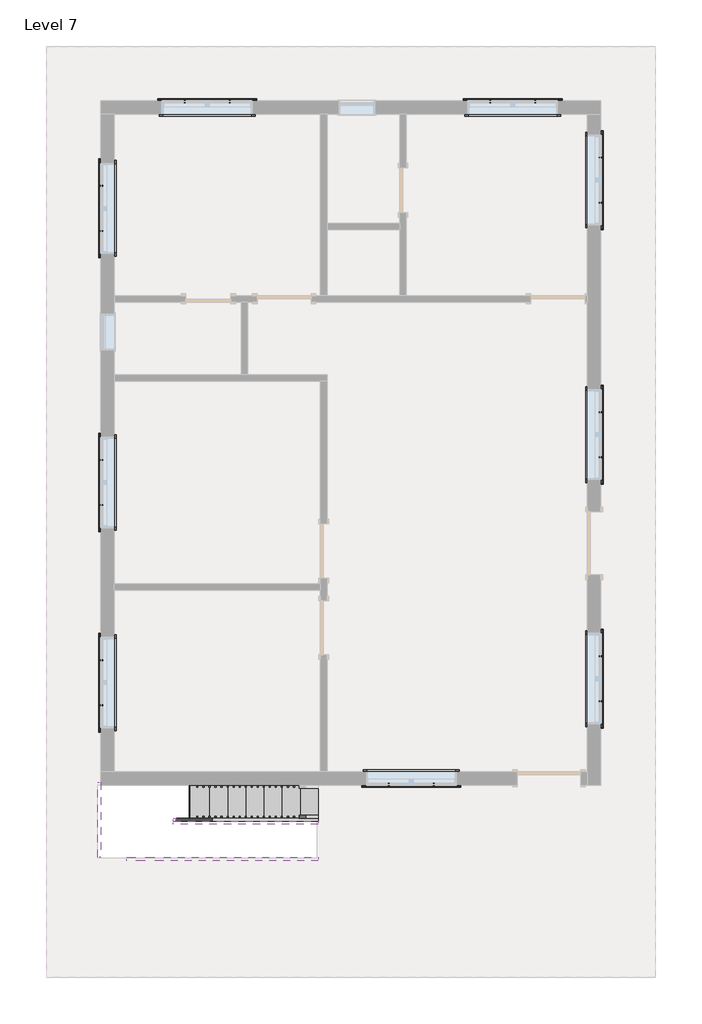
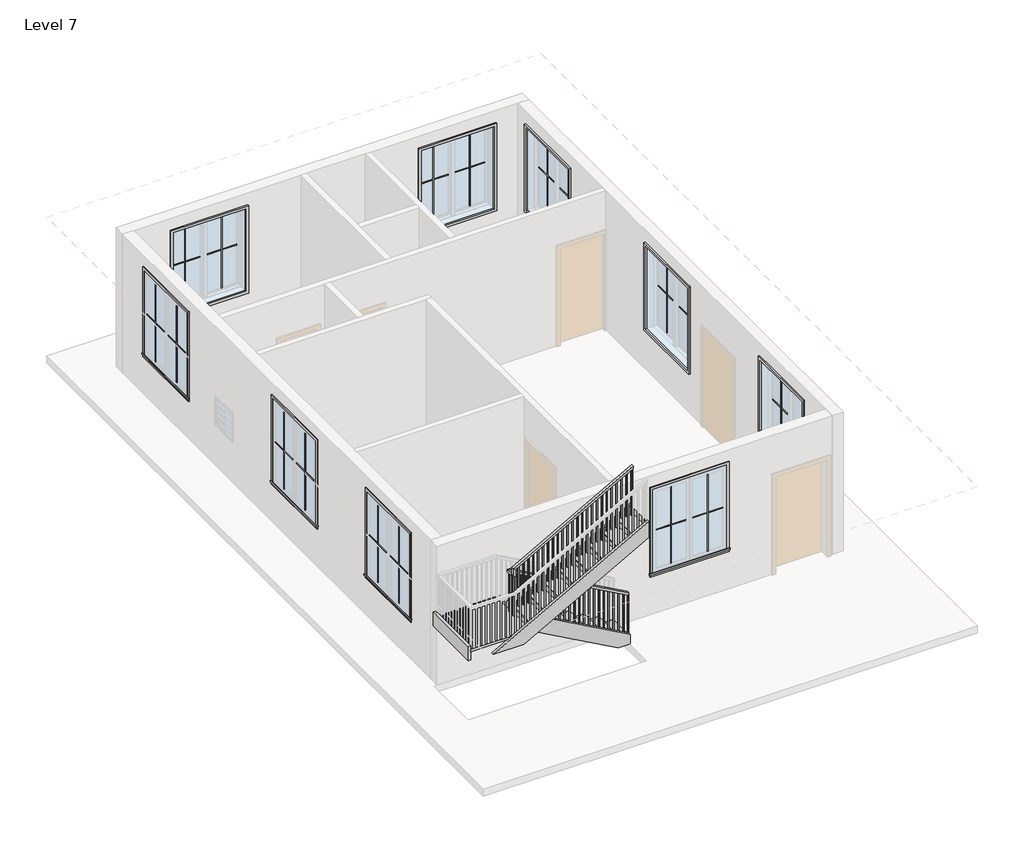
# One storey, part 3 of 3: 36 proxies, 6 members, 1 railing, 1 stair flight.
"""IFC4 building model written with IfcOpenShell, lengths in millimetres."""

from ifc_helpers import new_model, si_unit, frame, origin, place, context, project, spatial, polyline, outline, extrude, faceted_brep, transform, mapped, element, save
from components import muntin_pattern_2x2_muntin_pattern_2x2_f6a80940, muntin_pattern_2x2_muntin_pattern_2x2_09b00a1c, trim_window_exterior_flat_with_sill_698ed857, trim_window_interior_flat_picture_frame_92551a5e, stair_flight_b2054cc5

model = new_model("IFC4")

# Units and contexts
model_context = context("Model", 3, world=origin())
ifc_project = project(units=[si_unit("LENGTHUNIT", "METRE", prefix="MILLI")], contexts=[model_context])

# Site, building, storey
site = spatial("IfcSite", under=ifc_project)
building = spatial("IfcBuilding", under=site)
storey = spatial("IfcBuildingStorey", under=building, Name="Level 7", Elevation=16002.0)

# Proxies
placement = place(None, origin())
muntin_pattern_2x2_muntin_pattern_2x2_shape = muntin_pattern_2x2_muntin_pattern_2x2_f6a80940(model_context)
element("IfcBuildingElementProxy", 1, Name="Muntin Pattern_2x2 : Muntin Pattern_2x2", ObjectType="Muntin Pattern_2x2 : Muntin Pattern_2x2", at=placement, inside=storey, context=model_context, shape_type="MappedRepresentation", body=[
    mapped(muntin_pattern_2x2_muntin_pattern_2x2_shape, transform((-5453.9948569, -3961.7808037, 16986.25), x_axis=(0.0, 1.0, 0.0), y_axis=(-1.0, 0.0, 0.0), z_axis=(0.0, 0.0, 1.0))),
])
element("IfcBuildingElementProxy", 2, Name="Muntin Pattern_2x2 : Muntin Pattern_2x2", ObjectType="Muntin Pattern_2x2 : Muntin Pattern_2x2", at=placement, inside=storey, context=model_context, shape_type="MappedRepresentation", body=[
    mapped(muntin_pattern_2x2_muntin_pattern_2x2_shape, transform((-5453.9948569, -593.1058037, 16986.25), x_axis=(0.0, 1.0, 0.0), y_axis=(-1.0, 0.0, 0.0), z_axis=(0.0, 0.0, 1.0))),
])
element("IfcBuildingElementProxy", 3, Name="Muntin Pattern_2x2 : Muntin Pattern_2x2", ObjectType="Muntin Pattern_2x2 : Muntin Pattern_2x2", at=placement, inside=storey, context=model_context, shape_type="MappedRepresentation", body=[
    mapped(muntin_pattern_2x2_muntin_pattern_2x2_shape, transform((-5453.9948569, 4023.3441963, 16986.25), x_axis=(0.0, 1.0, 0.0), y_axis=(-1.0, 0.0, 0.0), z_axis=(0.0, 0.0, 1.0))),
])
element("IfcBuildingElementProxy", 4, Name="Muntin Pattern_2x2 : Muntin Pattern_2x2", ObjectType="Muntin Pattern_2x2 : Muntin Pattern_2x2", at=placement, inside=storey, context=model_context, shape_type="MappedRepresentation", body=[
    mapped(muntin_pattern_2x2_muntin_pattern_2x2_shape, transform((2947.0551431, 5258.4191963, 16986.25), x_axis=(0.0, -1.0, 0.0), y_axis=(1.0, 0.0, 0.0), z_axis=(0.0, 0.0, 1.0))),
])
element("IfcBuildingElementProxy", 5, Name="Muntin Pattern_2x2 : Muntin Pattern_2x2", ObjectType="Muntin Pattern_2x2 : Muntin Pattern_2x2", at=placement, inside=storey, context=model_context, shape_type="MappedRepresentation", body=[
    mapped(muntin_pattern_2x2_muntin_pattern_2x2_shape, transform((2947.0551431, 972.1691963, 16986.25), x_axis=(0.0, -1.0, 0.0), y_axis=(1.0, 0.0, 0.0), z_axis=(0.0, 0.0, 1.0))),
])
element("IfcBuildingElementProxy", 6, Name="Muntin Pattern_2x2 : Muntin Pattern_2x2", ObjectType="Muntin Pattern_2x2 : Muntin Pattern_2x2", at=placement, inside=storey, context=model_context, shape_type="MappedRepresentation", body=[
    mapped(muntin_pattern_2x2_muntin_pattern_2x2_shape, transform((2947.0551431, -3136.2808037, 16986.25), x_axis=(0.0, -1.0, 0.0), y_axis=(1.0, 0.0, 0.0), z_axis=(0.0, 0.0, 1.0))),
])
element("IfcBuildingElementProxy", 7, Name="Muntin Pattern_2x2 : Muntin Pattern_2x2", ObjectType="Muntin Pattern_2x2 : Muntin Pattern_2x2", at=placement, inside=storey, context=model_context, shape_type="MappedRepresentation", body=[
    mapped(muntin_pattern_2x2_muntin_pattern_2x2_shape, transform((141.9426431, -5296.8683037, 16986.25), x_axis=(-1.0, 0.0, 0.0), y_axis=(0.0, -1.0, 0.0), z_axis=(0.0, 0.0, 1.0))),
])
element("IfcBuildingElementProxy", 8, Name="Muntin Pattern_2x2 : Muntin Pattern_2x2", ObjectType="Muntin Pattern_2x2 : Muntin Pattern_2x2", at=placement, inside=storey, context=model_context, shape_type="MappedRepresentation", body=[
    mapped(muntin_pattern_2x2_muntin_pattern_2x2_shape, transform((1091.2676431, 6202.9816963, 16986.25), x_axis=(1.0, 0.0, 0.0), y_axis=(0.0, 1.0, 0.0), z_axis=(0.0, 0.0, 1.0))),
])
element("IfcBuildingElementProxy", 9, Name="Muntin Pattern_2x2 : Muntin Pattern_2x2", ObjectType="Muntin Pattern_2x2 : Muntin Pattern_2x2", at=placement, inside=storey, context=model_context, shape_type="MappedRepresentation", body=[
    mapped(muntin_pattern_2x2_muntin_pattern_2x2_shape, transform((-4052.2323569, 6202.9816963, 16986.25), x_axis=(1.0, 0.0, 0.0), y_axis=(0.0, 1.0, 0.0), z_axis=(0.0, 0.0, 1.0))),
])
muntin_pattern_2x2_muntin_pattern_2x2_2_shape = muntin_pattern_2x2_muntin_pattern_2x2_09b00a1c(model_context)
element("IfcBuildingElementProxy", 10, Name="Muntin Pattern_2x2 : Muntin Pattern_2x2", ObjectType="Muntin Pattern_2x2 : Muntin Pattern_2x2", at=placement, inside=storey, context=model_context, shape_type="MappedRepresentation", body=[
    mapped(muntin_pattern_2x2_muntin_pattern_2x2_2_shape, transform((-5453.9948569, -3202.9558037, 16986.25), x_axis=(0.0, -1.0, 0.0), y_axis=(1.0, 0.0, 0.0), z_axis=(0.0, 0.0, 1.0))),
])
element("IfcBuildingElementProxy", 11, Name="Muntin Pattern_2x2 : Muntin Pattern_2x2", ObjectType="Muntin Pattern_2x2 : Muntin Pattern_2x2", at=placement, inside=storey, context=model_context, shape_type="MappedRepresentation", body=[
    mapped(muntin_pattern_2x2_muntin_pattern_2x2_2_shape, transform((-5453.9948569, 165.7191963, 16986.25), x_axis=(0.0, -1.0, 0.0), y_axis=(1.0, 0.0, 0.0), z_axis=(0.0, 0.0, 1.0))),
])
element("IfcBuildingElementProxy", 12, Name="Muntin Pattern_2x2 : Muntin Pattern_2x2", ObjectType="Muntin Pattern_2x2 : Muntin Pattern_2x2", at=placement, inside=storey, context=model_context, shape_type="MappedRepresentation", body=[
    mapped(muntin_pattern_2x2_muntin_pattern_2x2_2_shape, transform((-5453.9948569, 4782.1691963, 16986.25), x_axis=(0.0, -1.0, 0.0), y_axis=(1.0, 0.0, 0.0), z_axis=(0.0, 0.0, 1.0))),
])
element("IfcBuildingElementProxy", 13, Name="Muntin Pattern_2x2 : Muntin Pattern_2x2", ObjectType="Muntin Pattern_2x2 : Muntin Pattern_2x2", at=placement, inside=storey, context=model_context, shape_type="MappedRepresentation", body=[
    mapped(muntin_pattern_2x2_muntin_pattern_2x2_2_shape, transform((2947.0551431, 4499.5941963, 16986.25), x_axis=(0.0, 1.0, 0.0), y_axis=(-1.0, 0.0, 0.0), z_axis=(0.0, 0.0, 1.0))),
])
element("IfcBuildingElementProxy", 14, Name="Muntin Pattern_2x2 : Muntin Pattern_2x2", ObjectType="Muntin Pattern_2x2 : Muntin Pattern_2x2", at=placement, inside=storey, context=model_context, shape_type="MappedRepresentation", body=[
    mapped(muntin_pattern_2x2_muntin_pattern_2x2_2_shape, transform((2947.0551431, 213.3441963, 16986.25), x_axis=(0.0, 1.0, 0.0), y_axis=(-1.0, 0.0, 0.0), z_axis=(0.0, 0.0, 1.0))),
])
element("IfcBuildingElementProxy", 15, Name="Muntin Pattern_2x2 : Muntin Pattern_2x2", ObjectType="Muntin Pattern_2x2 : Muntin Pattern_2x2", at=placement, inside=storey, context=model_context, shape_type="MappedRepresentation", body=[
    mapped(muntin_pattern_2x2_muntin_pattern_2x2_2_shape, transform((2947.0551431, -3895.1058037, 16986.25), x_axis=(0.0, 1.0, 0.0), y_axis=(-1.0, 0.0, 0.0), z_axis=(0.0, 0.0, 1.0))),
])
element("IfcBuildingElementProxy", 16, Name="Muntin Pattern_2x2 : Muntin Pattern_2x2", ObjectType="Muntin Pattern_2x2 : Muntin Pattern_2x2", at=placement, inside=storey, context=model_context, shape_type="MappedRepresentation", body=[
    mapped(muntin_pattern_2x2_muntin_pattern_2x2_2_shape, transform((-616.8823569, -5296.8683037, 16986.25), x_axis=(1.0, 0.0, 0.0), y_axis=(0.0, 1.0, 0.0), z_axis=(0.0, 0.0, 1.0))),
])
element("IfcBuildingElementProxy", 17, Name="Muntin Pattern_2x2 : Muntin Pattern_2x2", ObjectType="Muntin Pattern_2x2 : Muntin Pattern_2x2", at=placement, inside=storey, context=model_context, shape_type="MappedRepresentation", body=[
    mapped(muntin_pattern_2x2_muntin_pattern_2x2_2_shape, transform((1850.0926431, 6202.9816963, 16986.25), x_axis=(-1.0, 0.0, 0.0), y_axis=(0.0, -1.0, 0.0), z_axis=(0.0, 0.0, 1.0))),
])
element("IfcBuildingElementProxy", 18, Name="Muntin Pattern_2x2 : Muntin Pattern_2x2", ObjectType="Muntin Pattern_2x2 : Muntin Pattern_2x2", at=placement, inside=storey, context=model_context, shape_type="MappedRepresentation", body=[
    mapped(muntin_pattern_2x2_muntin_pattern_2x2_2_shape, transform((-3293.4073569, 6202.9816963, 16986.25), x_axis=(-1.0, 0.0, 0.0), y_axis=(0.0, -1.0, 0.0), z_axis=(0.0, 0.0, 1.0))),
])
trim_window_exterior_flat_with_sill_shape = trim_window_exterior_flat_with_sill_698ed857(model_context)
element("IfcBuildingElementProxy", 19, Name="Trim-Window-Exterior-Flat : with Sill", ObjectType="Trim-Window-Exterior-Flat : with Sill", at=placement, inside=storey, context=model_context, shape_type="MappedRepresentation", body=[
    mapped(trim_window_exterior_flat_with_sill_shape, transform((-5463.5198569, -3582.3683037, 18745.2), x_axis=(0.0, -1.0, 0.0), y_axis=(0.0, 0.0, 1.0), z_axis=(-1.0, 0.0, 0.0))),
])
element("IfcBuildingElementProxy", 20, Name="Trim-Window-Exterior-Flat : with Sill", ObjectType="Trim-Window-Exterior-Flat : with Sill", at=placement, inside=storey, context=model_context, shape_type="MappedRepresentation", body=[
    mapped(trim_window_exterior_flat_with_sill_shape, transform((-5463.5198569, -213.6933037, 18745.2), x_axis=(0.0, -1.0, 0.0), y_axis=(0.0, 0.0, 1.0), z_axis=(-1.0, 0.0, 0.0))),
])
element("IfcBuildingElementProxy", 21, Name="Trim-Window-Exterior-Flat : with Sill", ObjectType="Trim-Window-Exterior-Flat : with Sill", at=placement, inside=storey, context=model_context, shape_type="MappedRepresentation", body=[
    mapped(trim_window_exterior_flat_with_sill_shape, transform((-5463.5198569, 4402.7566963, 18745.2), x_axis=(0.0, -1.0, 0.0), y_axis=(0.0, 0.0, 1.0), z_axis=(-1.0, 0.0, 0.0))),
])
element("IfcBuildingElementProxy", 22, Name="Trim-Window-Exterior-Flat : with Sill", ObjectType="Trim-Window-Exterior-Flat : with Sill", at=placement, inside=storey, context=model_context, shape_type="MappedRepresentation", body=[
    mapped(trim_window_exterior_flat_with_sill_shape, transform((2956.5801431, 4879.0066963, 18745.2), x_axis=(0.0, 1.0, 0.0), y_axis=(0.0, 0.0, 1.0), z_axis=(1.0, 0.0, 0.0))),
])
element("IfcBuildingElementProxy", 23, Name="Trim-Window-Exterior-Flat : with Sill", ObjectType="Trim-Window-Exterior-Flat : with Sill", at=placement, inside=storey, context=model_context, shape_type="MappedRepresentation", body=[
    mapped(trim_window_exterior_flat_with_sill_shape, transform((2956.5801431, 592.7566963, 18745.2), x_axis=(0.0, 1.0, 0.0), y_axis=(0.0, 0.0, 1.0), z_axis=(1.0, 0.0, 0.0))),
])
element("IfcBuildingElementProxy", 24, Name="Trim-Window-Exterior-Flat : with Sill", ObjectType="Trim-Window-Exterior-Flat : with Sill", at=placement, inside=storey, context=model_context, shape_type="MappedRepresentation", body=[
    mapped(trim_window_exterior_flat_with_sill_shape, transform((2956.5801431, -3515.6933037, 18745.2), x_axis=(0.0, 1.0, 0.0), y_axis=(0.0, 0.0, 1.0), z_axis=(1.0, 0.0, 0.0))),
])
element("IfcBuildingElementProxy", 25, Name="Trim-Window-Exterior-Flat : with Sill", ObjectType="Trim-Window-Exterior-Flat : with Sill", at=placement, inside=storey, context=model_context, shape_type="MappedRepresentation", body=[
    mapped(trim_window_exterior_flat_with_sill_shape, transform((-237.4698569, -5306.3933037, 18745.2), x_axis=(1.0, 0.0, 0.0), y_axis=(0.0, 0.0, 1.0), z_axis=(0.0, -1.0, 0.0))),
])
element("IfcBuildingElementProxy", 26, Name="Trim-Window-Exterior-Flat : with Sill", ObjectType="Trim-Window-Exterior-Flat : with Sill", at=placement, inside=storey, context=model_context, shape_type="MappedRepresentation", body=[
    mapped(trim_window_exterior_flat_with_sill_shape, transform((1470.6801431, 6212.5066963, 18745.2), x_axis=(-1.0, 0.0, 0.0), y_axis=(0.0, 0.0, 1.0), z_axis=(0.0, 1.0, 0.0))),
])
element("IfcBuildingElementProxy", 27, Name="Trim-Window-Exterior-Flat : with Sill", ObjectType="Trim-Window-Exterior-Flat : with Sill", at=placement, inside=storey, context=model_context, shape_type="MappedRepresentation", body=[
    mapped(trim_window_exterior_flat_with_sill_shape, transform((-3672.8198569, 6212.5066963, 18745.2), x_axis=(-1.0, 0.0, 0.0), y_axis=(0.0, 0.0, 1.0), z_axis=(0.0, 1.0, 0.0))),
])
trim_window_interior_flat_picture_frame_shape = trim_window_interior_flat_picture_frame_92551a5e(model_context)
element("IfcBuildingElementProxy", 28, Name="Trim-Window-Interior-Flat : Picture Frame", ObjectType="Trim-Window-Interior-Flat : Picture Frame", at=placement, inside=storey, context=model_context, shape_type="MappedRepresentation", body=[
    mapped(trim_window_interior_flat_picture_frame_shape, transform((-5234.9198569, -3582.3683037, 18745.2), x_axis=(0.0, 1.0, 0.0), y_axis=(0.0, 0.0, 1.0), z_axis=(1.0, 0.0, 0.0))),
])
element("IfcBuildingElementProxy", 29, Name="Trim-Window-Interior-Flat : Picture Frame", ObjectType="Trim-Window-Interior-Flat : Picture Frame", at=placement, inside=storey, context=model_context, shape_type="MappedRepresentation", body=[
    mapped(trim_window_interior_flat_picture_frame_shape, transform((-5234.9198569, -213.6933037, 18745.2), x_axis=(0.0, 1.0, 0.0), y_axis=(0.0, 0.0, 1.0), z_axis=(1.0, 0.0, 0.0))),
])
element("IfcBuildingElementProxy", 30, Name="Trim-Window-Interior-Flat : Picture Frame", ObjectType="Trim-Window-Interior-Flat : Picture Frame", at=placement, inside=storey, context=model_context, shape_type="MappedRepresentation", body=[
    mapped(trim_window_interior_flat_picture_frame_shape, transform((-5234.9198569, 4402.7566963, 18745.2), x_axis=(0.0, 1.0, 0.0), y_axis=(0.0, 0.0, 1.0), z_axis=(1.0, 0.0, 0.0))),
])
element("IfcBuildingElementProxy", 31, Name="Trim-Window-Interior-Flat : Picture Frame", ObjectType="Trim-Window-Interior-Flat : Picture Frame", at=placement, inside=storey, context=model_context, shape_type="MappedRepresentation", body=[
    mapped(trim_window_interior_flat_picture_frame_shape, transform((2727.9801431, 4879.0066963, 18745.2), x_axis=(0.0, -1.0, 0.0), y_axis=(0.0, 0.0, 1.0), z_axis=(-1.0, 0.0, 0.0))),
])
element("IfcBuildingElementProxy", 32, Name="Trim-Window-Interior-Flat : Picture Frame", ObjectType="Trim-Window-Interior-Flat : Picture Frame", at=placement, inside=storey, context=model_context, shape_type="MappedRepresentation", body=[
    mapped(trim_window_interior_flat_picture_frame_shape, transform((2727.9801431, 592.7566963, 18745.2), x_axis=(0.0, -1.0, 0.0), y_axis=(0.0, 0.0, 1.0), z_axis=(-1.0, 0.0, 0.0))),
])
element("IfcBuildingElementProxy", 33, Name="Trim-Window-Interior-Flat : Picture Frame", ObjectType="Trim-Window-Interior-Flat : Picture Frame", at=placement, inside=storey, context=model_context, shape_type="MappedRepresentation", body=[
    mapped(trim_window_interior_flat_picture_frame_shape, transform((2727.9801431, -3515.6933037, 18745.2), x_axis=(0.0, -1.0, 0.0), y_axis=(0.0, 0.0, 1.0), z_axis=(-1.0, 0.0, 0.0))),
])
element("IfcBuildingElementProxy", 34, Name="Trim-Window-Interior-Flat : Picture Frame", ObjectType="Trim-Window-Interior-Flat : Picture Frame", at=placement, inside=storey, context=model_context, shape_type="MappedRepresentation", body=[
    mapped(trim_window_interior_flat_picture_frame_shape, transform((-237.4698569, -5077.7933037, 18745.2), x_axis=(-1.0, 0.0, 0.0), y_axis=(0.0, 0.0, 1.0), z_axis=(0.0, 1.0, 0.0))),
])
element("IfcBuildingElementProxy", 35, Name="Trim-Window-Interior-Flat : Picture Frame", ObjectType="Trim-Window-Interior-Flat : Picture Frame", at=placement, inside=storey, context=model_context, shape_type="MappedRepresentation", body=[
    mapped(trim_window_interior_flat_picture_frame_shape, transform((1470.6801431, 5983.9066963, 18745.2), x_axis=(1.0, 0.0, 0.0), y_axis=(0.0, 0.0, 1.0), z_axis=(0.0, -1.0, 0.0))),
])
element("IfcBuildingElementProxy", 36, Name="Trim-Window-Interior-Flat : Picture Frame", ObjectType="Trim-Window-Interior-Flat : Picture Frame", at=placement, inside=storey, context=model_context, shape_type="MappedRepresentation", body=[
    mapped(trim_window_interior_flat_picture_frame_shape, transform((-3672.8198569, 5983.9066963, 18745.2), x_axis=(1.0, 0.0, 0.0), y_axis=(0.0, 0.0, 1.0), z_axis=(0.0, -1.0, 0.0))),
])

# Members
element("IfcMember", 37, ObjectType="Stringer - 2\" Width", at=placement, inside=storey, context=model_context, shape_type="SweptSolid", body=[
    extrude(outline(polyline([(16002.0, -1805.9198569), (16209.5983948, -1805.9198569), (17536.0428392, -4193.5198569), (17187.3641651, -4193.5198569), (16002.0, -2059.8643597), (16002.0, -1805.9198569)])), frame((0.0, -5915.9933037, 0.0), z_axis=(0.0, 1.0, 0.0), x_axis=(0.0, 0.0, 1.0)), (0.0, 0.0, 1.0), 50.8),
])
element("IfcMember", 38, ObjectType="Stringer - 2\" Width", at=placement, inside=storey, context=model_context, shape_type="SweptSolid", body=[
    extrude(outline(polyline([(-4244.3198569, -5865.1933037), (-4193.5198569, -5865.1933037), (-4193.5198569, -5915.9933037), (-4244.3198569, -5915.9933037), (-4244.3198569, -5865.1933037)])), frame((0.0, 0.0, 17297.4), z_axis=(0.0, 0.0, 1.0), x_axis=(1.0, 0.0, 0.0)), (0.0, 0.0, 1.0), 304.8),
])
element("IfcMember", 39, ObjectType="Stringer - 2\" Width", at=placement, inside=storey, context=model_context, shape_type="SweptSolid", body=[
    extrude(outline(polyline([(17733.5983948, -4244.3198569), (17384.9197207, -4244.3198569), (18739.5863873, -1805.9198569), (19088.2650614, -1805.9198569), (17733.5983948, -4244.3198569)])), frame((0.0, -5966.7933037, 0.0), z_axis=(0.0, 1.0, 0.0), x_axis=(0.0, 0.0, 1.0)), (0.0, 0.0, 1.0), 50.8),
])
element("IfcMember", 40, ObjectType="Stringer - 2\" Width", at=placement, inside=storey, context=model_context, shape_type="SweptSolid", body=[
    extrude(outline(polyline([(16002.0, -1805.9198569), (16209.5983948, -1805.9198569), (17602.2, -4312.6027463), (17602.2, -4940.2243597), (16002.0, -2059.8643597), (16002.0, -1805.9198569)])), frame((0.0, -5306.3933037, 0.0), z_axis=(0.0, 1.0, 0.0), x_axis=(0.0, 0.0, 1.0)), (0.0, 0.0, 1.0), 50.8),
])
element("IfcMember", 41, ObjectType="Stringer - 2\" Width", at=placement, inside=storey, context=model_context, shape_type="SweptSolid", body=[
    extrude(outline(polyline([(-5514.3198569, -5255.5933037), (-5463.5198569, -5255.5933037), (-5463.5198569, -6525.5933037), (-5514.3198569, -6525.5933037), (-5514.3198569, -5255.5933037)])), frame((0.0, 0.0, 17297.4), z_axis=(0.0, 0.0, 1.0), x_axis=(1.0, 0.0, 0.0)), (0.0, 0.0, 1.0), 304.8),
])
element("IfcMember", 42, ObjectType="Stringer - 2\" Width", at=placement, inside=storey, context=model_context, shape_type="SweptSolid", body=[
    extrude(outline(polyline([(17297.4, -4401.8553541), (18739.5863873, -1805.9198569), (19088.2650614, -1805.9198569), (17297.4, -5029.4769675), (17297.4, -4401.8553541)])), frame((0.0, -6576.3933037, 0.0), z_axis=(0.0, 1.0, 0.0), x_axis=(0.0, 0.0, 1.0)), (0.0, 0.0, 1.0), 50.8),
])

# Railing
element("IfcRailing", 43, ObjectType="Handrail - Rectangular", at=placement, inside=storey, context=model_context, shape_type="SolidModel", body=[
    faceted_brep([(-1805.9198569, -5865.1933037, 17085.7333333), (-1805.9198569, -5865.1933037, 17027.620221), (-1805.9198569, -5814.3933037, 17027.620221), (-1805.9198569, -5814.3933037, 17085.7333333), (-4168.1198569, -5865.1933037, 18398.0666667), (-4218.9198569, -5865.1933037, 18368.1757765), (-4218.9198569, -5814.3933037, 18368.1757765), (-4168.1198569, -5814.3933037, 18398.0666667), (-4168.1198569, -5865.1933037, 18440.4), (-4218.9198569, -5865.1933037, 18389.6), (-4218.9198569, -5814.3933037, 18389.6), (-4168.1198569, -5814.3933037, 18440.4), (-4244.3198569, -5865.1933037, 18440.4), (-4244.3198569, -5865.1933037, 18389.6), (-4295.1198569, -5814.3933037, 18389.6), (-4295.1198569, -5814.3933037, 18440.4), (-4244.3198569, -5941.3933037, 18440.4), (-4244.3198569, -5941.3933037, 18389.6), (-4295.1198569, -5941.3933037, 18389.6), (-4295.1198569, -5941.3933037, 18440.4), (-4244.3198569, -5966.7933037, 18440.4), (-4295.1198569, -5966.7933037, 18440.4), (-4295.1198569, -6017.5933037, 18389.6), (-4244.3198569, -6017.5933037, 18389.6)], [[[0, 1, 2, 3]], [[1, 0, 4, 5]], [[2, 1, 5, 6]], [[3, 2, 6, 7]], [[0, 3, 7, 4]], [[5, 4, 8, 9]], [[6, 5, 9, 10]], [[7, 6, 10, 11]], [[4, 7, 11, 8]], [[9, 8, 12, 13]], [[10, 9, 13, 14]], [[11, 10, 14, 15]], [[8, 11, 15, 12]], [[13, 12, 16, 17]], [[14, 13, 17, 18]], [[15, 14, 18, 19]], [[12, 15, 19, 16]], [[20, 21, 22, 23]], [[17, 16, 20, 23]], [[18, 17, 23, 22]], [[19, 18, 22, 21]], [[16, 19, 21, 20]]]),
    faceted_brep([(-4244.3198569, -5966.7933037, 18440.4), (-4244.3198569, -6017.5933037, 18389.6), (-4295.1198569, -6017.5933037, 18389.6), (-4295.1198569, -5966.7933037, 18440.4), (-4244.3198569, -5966.7933037, 18551.620221), (-4295.1198569, -5966.7933037, 18581.5111111), (-4295.1198569, -6017.5933037, 18581.5111111), (-4244.3198569, -6017.5933037, 18551.620221)], [[[0, 1, 2, 3]], [[4, 5, 6, 7]], [[1, 0, 4, 7]], [[2, 1, 7, 6]], [[3, 2, 6, 5]], [[0, 3, 5, 4]]]),
    faceted_brep([(-4295.1198569, -5966.7933037, 18581.5111111), (-4244.3198569, -5966.7933037, 18551.620221), (-4244.3198569, -6017.5933037, 18551.620221), (-4295.1198569, -6017.5933037, 18581.5111111), (-1805.9198569, -5966.7933037, 19964.4), (-1805.9198569, -6017.5933037, 19964.4), (-1805.9198569, -6017.5933037, 19906.2868876), (-1805.9198569, -5966.7933037, 19906.2868876)], [[[0, 1, 2, 3]], [[4, 5, 6, 7]], [[1, 0, 4, 7]], [[2, 1, 7, 6]], [[3, 2, 6, 5]], [[0, 3, 5, 4]]]),
    extrude(outline(polyline([(19886.8841099, -1840.8448569), (18880.6666667, -1840.8448569), (18880.6666667, -1821.7948569), (19897.4674432, -1821.7948569), (19886.8841099, -1840.8448569)])), frame((0.0, -6001.7183037, 0.0), z_axis=(0.0, 1.0, 0.0), x_axis=(0.0, 0.0, 1.0)), (0.0, 0.0, 1.0), 19.05),
    extrude(outline(polyline([(19830.4396654, -1942.4448569), (18880.6666667, -1942.4448569), (18880.6666667, -1923.3948569), (19841.0229988, -1923.3948569), (19830.4396654, -1942.4448569)])), frame((0.0, -6001.7183037, 0.0), z_axis=(0.0, 1.0, 0.0), x_axis=(0.0, 0.0, 1.0)), (0.0, 0.0, 1.0), 19.05),
    extrude(outline(polyline([(19773.995221, -2044.0448569), (18880.6666667, -2044.0448569), (18880.6666667, -2024.9948569), (19784.5785543, -2024.9948569), (19773.995221, -2044.0448569)])), frame((0.0, -6001.7183037, 0.0), z_axis=(0.0, 1.0, 0.0), x_axis=(0.0, 0.0, 1.0)), (0.0, 0.0, 1.0), 19.05),
    extrude(outline(polyline([(19717.5507765, -2145.6448569), (18711.3333333, -2145.6448569), (18711.3333333, -2126.5948569), (19728.1341099, -2126.5948569), (19717.5507765, -2145.6448569)])), frame((0.0, -6001.7183037, 0.0), z_axis=(0.0, 1.0, 0.0), x_axis=(0.0, 0.0, 1.0)), (0.0, 0.0, 1.0), 19.05),
    extrude(outline(polyline([(19661.1063321, -2247.2448569), (18711.3333333, -2247.2448569), (18711.3333333, -2228.1948569), (19671.6896654, -2228.1948569), (19661.1063321, -2247.2448569)])), frame((0.0, -6001.7183037, 0.0), z_axis=(0.0, 1.0, 0.0), x_axis=(0.0, 0.0, 1.0)), (0.0, 0.0, 1.0), 19.05),
    extrude(outline(polyline([(19604.6618876, -2348.8448569), (18711.3333333, -2348.8448569), (18711.3333333, -2329.7948569), (19615.245221, -2329.7948569), (19604.6618876, -2348.8448569)])), frame((0.0, -6001.7183037, 0.0), z_axis=(0.0, 1.0, 0.0), x_axis=(0.0, 0.0, 1.0)), (0.0, 0.0, 1.0), 19.05),
    extrude(outline(polyline([(19548.2174432, -2450.4448569), (18542.0, -2450.4448569), (18542.0, -2431.3948569), (19558.8007765, -2431.3948569), (19548.2174432, -2450.4448569)])), frame((0.0, -6001.7183037, 0.0), z_axis=(0.0, 1.0, 0.0), x_axis=(0.0, 0.0, 1.0)), (0.0, 0.0, 1.0), 19.05),
    extrude(outline(polyline([(19491.7729988, -2552.0448569), (18542.0, -2552.0448569), (18542.0, -2532.9948569), (19502.3563321, -2532.9948569), (19491.7729988, -2552.0448569)])), frame((0.0, -6001.7183037, 0.0), z_axis=(0.0, 1.0, 0.0), x_axis=(0.0, 0.0, 1.0)), (0.0, 0.0, 1.0), 19.05),
    extrude(outline(polyline([(19435.3285543, -2653.6448569), (18542.0, -2653.6448569), (18542.0, -2634.5948569), (19445.9118876, -2634.5948569), (19435.3285543, -2653.6448569)])), frame((0.0, -6001.7183037, 0.0), z_axis=(0.0, 1.0, 0.0), x_axis=(0.0, 0.0, 1.0)), (0.0, 0.0, 1.0), 19.05),
    extrude(outline(polyline([(19378.8841099, -2755.2448569), (18372.6666667, -2755.2448569), (18372.6666667, -2736.1948569), (19389.4674432, -2736.1948569), (19378.8841099, -2755.2448569)])), frame((0.0, -6001.7183037, 0.0), z_axis=(0.0, 1.0, 0.0), x_axis=(0.0, 0.0, 1.0)), (0.0, 0.0, 1.0), 19.05),
    extrude(outline(polyline([(19322.4396654, -2856.8448569), (18372.6666667, -2856.8448569), (18372.6666667, -2837.7948569), (19333.0229988, -2837.7948569), (19322.4396654, -2856.8448569)])), frame((0.0, -6001.7183037, 0.0), z_axis=(0.0, 1.0, 0.0), x_axis=(0.0, 0.0, 1.0)), (0.0, 0.0, 1.0), 19.05),
    extrude(outline(polyline([(19265.995221, -2958.4448569), (18372.6666667, -2958.4448569), (18372.6666667, -2939.3948569), (19276.5785543, -2939.3948569), (19265.995221, -2958.4448569)])), frame((0.0, -6001.7183037, 0.0), z_axis=(0.0, 1.0, 0.0), x_axis=(0.0, 0.0, 1.0)), (0.0, 0.0, 1.0), 19.05),
    extrude(outline(polyline([(19209.5507765, -3060.0448569), (18203.3333333, -3060.0448569), (18203.3333333, -3040.9948569), (19220.1341099, -3040.9948569), (19209.5507765, -3060.0448569)])), frame((0.0, -6001.7183037, 0.0), z_axis=(0.0, 1.0, 0.0), x_axis=(0.0, 0.0, 1.0)), (0.0, 0.0, 1.0), 19.05),
    extrude(outline(polyline([(19153.1063321, -3161.6448569), (18203.3333333, -3161.6448569), (18203.3333333, -3142.5948569), (19163.6896654, -3142.5948569), (19153.1063321, -3161.6448569)])), frame((0.0, -6001.7183037, 0.0), z_axis=(0.0, 1.0, 0.0), x_axis=(0.0, 0.0, 1.0)), (0.0, 0.0, 1.0), 19.05),
    extrude(outline(polyline([(19096.6618876, -3263.2448569), (18203.3333333, -3263.2448569), (18203.3333333, -3244.1948569), (19107.245221, -3244.1948569), (19096.6618876, -3263.2448569)])), frame((0.0, -6001.7183037, 0.0), z_axis=(0.0, 1.0, 0.0), x_axis=(0.0, 0.0, 1.0)), (0.0, 0.0, 1.0), 19.05),
    extrude(outline(polyline([(19040.2174432, -3364.8448569), (18034.0, -3364.8448569), (18034.0, -3345.7948569), (19050.8007765, -3345.7948569), (19040.2174432, -3364.8448569)])), frame((0.0, -6001.7183037, 0.0), z_axis=(0.0, 1.0, 0.0), x_axis=(0.0, 0.0, 1.0)), (0.0, 0.0, 1.0), 19.05),
    extrude(outline(polyline([(18983.7729988, -3466.4448569), (18034.0, -3466.4448569), (18034.0, -3447.3948569), (18994.3563321, -3447.3948569), (18983.7729988, -3466.4448569)])), frame((0.0, -6001.7183037, 0.0), z_axis=(0.0, 1.0, 0.0), x_axis=(0.0, 0.0, 1.0)), (0.0, 0.0, 1.0), 19.05),
    extrude(outline(polyline([(18927.3285543, -3568.0448569), (18034.0, -3568.0448569), (18034.0, -3548.9948569), (18937.9118876, -3548.9948569), (18927.3285543, -3568.0448569)])), frame((0.0, -6001.7183037, 0.0), z_axis=(0.0, 1.0, 0.0), x_axis=(0.0, 0.0, 1.0)), (0.0, 0.0, 1.0), 19.05),
    extrude(outline(polyline([(18870.8841099, -3669.6448569), (17864.6666667, -3669.6448569), (17864.6666667, -3650.5948569), (18881.4674432, -3650.5948569), (18870.8841099, -3669.6448569)])), frame((0.0, -6001.7183037, 0.0), z_axis=(0.0, 1.0, 0.0), x_axis=(0.0, 0.0, 1.0)), (0.0, 0.0, 1.0), 19.05),
    extrude(outline(polyline([(18814.4396654, -3771.2448569), (17864.6666667, -3771.2448569), (17864.6666667, -3752.1948569), (18825.0229988, -3752.1948569), (18814.4396654, -3771.2448569)])), frame((0.0, -6001.7183037, 0.0), z_axis=(0.0, 1.0, 0.0), x_axis=(0.0, 0.0, 1.0)), (0.0, 0.0, 1.0), 19.05),
    extrude(outline(polyline([(18757.995221, -3872.8448569), (17864.6666667, -3872.8448569), (17864.6666667, -3853.7948569), (18768.5785543, -3853.7948569), (18757.995221, -3872.8448569)])), frame((0.0, -6001.7183037, 0.0), z_axis=(0.0, 1.0, 0.0), x_axis=(0.0, 0.0, 1.0)), (0.0, 0.0, 1.0), 19.05),
    extrude(outline(polyline([(18701.5507765, -3974.4448569), (17695.3333333, -3974.4448569), (17695.3333333, -3955.3948569), (18712.1341099, -3955.3948569), (18701.5507765, -3974.4448569)])), frame((0.0, -6001.7183037, 0.0), z_axis=(0.0, 1.0, 0.0), x_axis=(0.0, 0.0, 1.0)), (0.0, 0.0, 1.0), 19.05),
    extrude(outline(polyline([(18645.1063321, -4076.0448569), (17695.3333333, -4076.0448569), (17695.3333333, -4056.9948569), (18655.6896654, -4056.9948569), (18645.1063321, -4076.0448569)])), frame((0.0, -6001.7183037, 0.0), z_axis=(0.0, 1.0, 0.0), x_axis=(0.0, 0.0, 1.0)), (0.0, 0.0, 1.0), 19.05),
    extrude(outline(polyline([(18588.6618876, -4177.6448569), (17695.3333333, -4177.6448569), (17695.3333333, -4158.5948569), (18599.245221, -4158.5948569), (18588.6618876, -4177.6448569)])), frame((0.0, -6001.7183037, 0.0), z_axis=(0.0, 1.0, 0.0), x_axis=(0.0, 0.0, 1.0)), (0.0, 0.0, 1.0), 19.05),
    extrude(outline(polyline([(-4260.1948569, -5931.8683037), (-4260.1948569, -5950.9183037), (-4279.2448569, -5950.9183037), (-4279.2448569, -5931.8683037), (-4260.1948569, -5931.8683037)])), frame((0.0, 0.0, 17526.0), z_axis=(0.0, 0.0, 1.0), x_axis=(1.0, 0.0, 0.0)), (0.0, 0.0, 1.0), 863.6),
    extrude(outline(polyline([(-4234.7948569, -5849.3183037), (-4253.8448569, -5849.3183037), (-4253.8448569, -5830.2683037), (-4234.7948569, -5830.2683037), (-4234.7948569, -5849.3183037)])), frame((0.0, 0.0, 17526.0), z_axis=(0.0, 0.0, 1.0), x_axis=(1.0, 0.0, 0.0)), (0.0, 0.0, 1.0), 863.6),
    extrude(outline(polyline([(18331.1341099, -4152.2448569), (17356.6666667, -4152.2448569), (17356.6666667, -4133.1948569), (18320.5507765, -4133.1948569), (18331.1341099, -4152.2448569)])), frame((0.0, -5849.3183037, 0.0), z_axis=(0.0, 1.0, 0.0), x_axis=(0.0, 0.0, 1.0)), (0.0, 0.0, 1.0), 19.05),
    extrude(outline(polyline([(18274.6896654, -4050.6448569), (17356.6666667, -4050.6448569), (17356.6666667, -4031.5948569), (18264.1063321, -4031.5948569), (18274.6896654, -4050.6448569)])), frame((0.0, -5849.3183037, 0.0), z_axis=(0.0, 1.0, 0.0), x_axis=(0.0, 0.0, 1.0)), (0.0, 0.0, 1.0), 19.05),
    extrude(outline(polyline([(18218.245221, -3949.0448569), (17356.6666667, -3949.0448569), (17356.6666667, -3929.9948569), (18207.6618876, -3929.9948569), (18218.245221, -3949.0448569)])), frame((0.0, -5849.3183037, 0.0), z_axis=(0.0, 1.0, 0.0), x_axis=(0.0, 0.0, 1.0)), (0.0, 0.0, 1.0), 19.05),
    extrude(outline(polyline([(18161.8007765, -3847.4448569), (17187.3333333, -3847.4448569), (17187.3333333, -3828.3948569), (18151.2174432, -3828.3948569), (18161.8007765, -3847.4448569)])), frame((0.0, -5849.3183037, 0.0), z_axis=(0.0, 1.0, 0.0), x_axis=(0.0, 0.0, 1.0)), (0.0, 0.0, 1.0), 19.05),
    extrude(outline(polyline([(18105.3563321, -3745.8448569), (17187.3333333, -3745.8448569), (17187.3333333, -3726.7948569), (18094.7729988, -3726.7948569), (18105.3563321, -3745.8448569)])), frame((0.0, -5849.3183037, 0.0), z_axis=(0.0, 1.0, 0.0), x_axis=(0.0, 0.0, 1.0)), (0.0, 0.0, 1.0), 19.05),
    extrude(outline(polyline([(18048.9118876, -3644.2448569), (17187.3333333, -3644.2448569), (17187.3333333, -3625.1948569), (18038.3285543, -3625.1948569), (18048.9118876, -3644.2448569)])), frame((0.0, -5849.3183037, 0.0), z_axis=(0.0, 1.0, 0.0), x_axis=(0.0, 0.0, 1.0)), (0.0, 0.0, 1.0), 19.05),
    extrude(outline(polyline([(17992.4674432, -3542.6448569), (17018.0, -3542.6448569), (17018.0, -3523.5948569), (17981.8841099, -3523.5948569), (17992.4674432, -3542.6448569)])), frame((0.0, -5849.3183037, 0.0), z_axis=(0.0, 1.0, 0.0), x_axis=(0.0, 0.0, 1.0)), (0.0, 0.0, 1.0), 19.05),
    extrude(outline(polyline([(17936.0229988, -3441.0448569), (17018.0, -3441.0448569), (17018.0, -3421.9948569), (17925.4396654, -3421.9948569), (17936.0229988, -3441.0448569)])), frame((0.0, -5849.3183037, 0.0), z_axis=(0.0, 1.0, 0.0), x_axis=(0.0, 0.0, 1.0)), (0.0, 0.0, 1.0), 19.05),
    extrude(outline(polyline([(17879.5785543, -3339.4448569), (17018.0, -3339.4448569), (17018.0, -3320.3948569), (17868.995221, -3320.3948569), (17879.5785543, -3339.4448569)])), frame((0.0, -5849.3183037, 0.0), z_axis=(0.0, 1.0, 0.0), x_axis=(0.0, 0.0, 1.0)), (0.0, 0.0, 1.0), 19.05),
    extrude(outline(polyline([(17823.1341099, -3237.8448569), (16848.6666667, -3237.8448569), (16848.6666667, -3218.7948569), (17812.5507765, -3218.7948569), (17823.1341099, -3237.8448569)])), frame((0.0, -5849.3183037, 0.0), z_axis=(0.0, 1.0, 0.0), x_axis=(0.0, 0.0, 1.0)), (0.0, 0.0, 1.0), 19.05),
    extrude(outline(polyline([(17766.6896654, -3136.2448569), (16848.6666667, -3136.2448569), (16848.6666667, -3117.1948569), (17756.1063321, -3117.1948569), (17766.6896654, -3136.2448569)])), frame((0.0, -5849.3183037, 0.0), z_axis=(0.0, 1.0, 0.0), x_axis=(0.0, 0.0, 1.0)), (0.0, 0.0, 1.0), 19.05),
    extrude(outline(polyline([(17710.245221, -3034.6448569), (16848.6666667, -3034.6448569), (16848.6666667, -3015.5948569), (17699.6618876, -3015.5948569), (17710.245221, -3034.6448569)])), frame((0.0, -5849.3183037, 0.0), z_axis=(0.0, 1.0, 0.0), x_axis=(0.0, 0.0, 1.0)), (0.0, 0.0, 1.0), 19.05),
    extrude(outline(polyline([(17653.8007765, -2933.0448569), (16679.3333333, -2933.0448569), (16679.3333333, -2913.9948569), (17643.2174432, -2913.9948569), (17653.8007765, -2933.0448569)])), frame((0.0, -5849.3183037, 0.0), z_axis=(0.0, 1.0, 0.0), x_axis=(0.0, 0.0, 1.0)), (0.0, 0.0, 1.0), 19.05),
    extrude(outline(polyline([(17597.3563321, -2831.4448569), (16679.3333333, -2831.4448569), (16679.3333333, -2812.3948569), (17586.7729988, -2812.3948569), (17597.3563321, -2831.4448569)])), frame((0.0, -5849.3183037, 0.0), z_axis=(0.0, 1.0, 0.0), x_axis=(0.0, 0.0, 1.0)), (0.0, 0.0, 1.0), 19.05),
    extrude(outline(polyline([(17540.9118876, -2729.8448569), (16679.3333333, -2729.8448569), (16679.3333333, -2710.7948569), (17530.3285543, -2710.7948569), (17540.9118876, -2729.8448569)])), frame((0.0, -5849.3183037, 0.0), z_axis=(0.0, 1.0, 0.0), x_axis=(0.0, 0.0, 1.0)), (0.0, 0.0, 1.0), 19.05),
    extrude(outline(polyline([(17484.4674432, -2628.2448569), (16510.0, -2628.2448569), (16510.0, -2609.1948569), (17473.8841099, -2609.1948569), (17484.4674432, -2628.2448569)])), frame((0.0, -5849.3183037, 0.0), z_axis=(0.0, 1.0, 0.0), x_axis=(0.0, 0.0, 1.0)), (0.0, 0.0, 1.0), 19.05),
    extrude(outline(polyline([(17428.0229988, -2526.6448569), (16510.0, -2526.6448569), (16510.0, -2507.5948569), (17417.4396654, -2507.5948569), (17428.0229988, -2526.6448569)])), frame((0.0, -5849.3183037, 0.0), z_axis=(0.0, 1.0, 0.0), x_axis=(0.0, 0.0, 1.0)), (0.0, 0.0, 1.0), 19.05),
    extrude(outline(polyline([(17371.5785543, -2425.0448569), (16510.0, -2425.0448569), (16510.0, -2405.9948569), (17360.995221, -2405.9948569), (17371.5785543, -2425.0448569)])), frame((0.0, -5849.3183037, 0.0), z_axis=(0.0, 1.0, 0.0), x_axis=(0.0, 0.0, 1.0)), (0.0, 0.0, 1.0), 19.05),
    extrude(outline(polyline([(17315.1341099, -2323.4448569), (16340.6666667, -2323.4448569), (16340.6666667, -2304.3948569), (17304.5507765, -2304.3948569), (17315.1341099, -2323.4448569)])), frame((0.0, -5849.3183037, 0.0), z_axis=(0.0, 1.0, 0.0), x_axis=(0.0, 0.0, 1.0)), (0.0, 0.0, 1.0), 19.05),
    extrude(outline(polyline([(17258.6896654, -2221.8448569), (16340.6666667, -2221.8448569), (16340.6666667, -2202.7948569), (17248.1063321, -2202.7948569), (17258.6896654, -2221.8448569)])), frame((0.0, -5849.3183037, 0.0), z_axis=(0.0, 1.0, 0.0), x_axis=(0.0, 0.0, 1.0)), (0.0, 0.0, 1.0), 19.05),
    extrude(outline(polyline([(17202.245221, -2120.2448569), (16340.6666667, -2120.2448569), (16340.6666667, -2101.1948569), (17191.6618876, -2101.1948569), (17202.245221, -2120.2448569)])), frame((0.0, -5849.3183037, 0.0), z_axis=(0.0, 1.0, 0.0), x_axis=(0.0, 0.0, 1.0)), (0.0, 0.0, 1.0), 19.05),
    extrude(outline(polyline([(17145.8007765, -2018.6448569), (16171.3333333, -2018.6448569), (16171.3333333, -1999.5948569), (17135.2174432, -1999.5948569), (17145.8007765, -2018.6448569)])), frame((0.0, -5849.3183037, 0.0), z_axis=(0.0, 1.0, 0.0), x_axis=(0.0, 0.0, 1.0)), (0.0, 0.0, 1.0), 19.05),
    extrude(outline(polyline([(17089.3563321, -1917.0448569), (16171.3333333, -1917.0448569), (16171.3333333, -1897.9948569), (17078.7729988, -1897.9948569), (17089.3563321, -1917.0448569)])), frame((0.0, -5849.3183037, 0.0), z_axis=(0.0, 1.0, 0.0), x_axis=(0.0, 0.0, 1.0)), (0.0, 0.0, 1.0), 19.05),
    extrude(outline(polyline([(-4260.1948569, -5982.6683037), (-4260.1948569, -6001.7183037), (-4279.2448569, -6001.7183037), (-4279.2448569, -5982.6683037), (-4260.1948569, -5982.6683037)])), frame((0.0, 0.0, 17526.0), z_axis=(0.0, 0.0, 1.0), x_axis=(1.0, 0.0, 0.0)), (0.0, 0.0, 1.0), 863.6),
    extrude(outline(polyline([(-4260.1948569, -5849.3183037), (-4279.2448569, -5849.3183037), (-4279.2448569, -5830.2683037), (-4260.1948569, -5830.2683037), (-4260.1948569, -5849.3183037)])), frame((0.0, 0.0, 17526.0), z_axis=(0.0, 0.0, 1.0), x_axis=(1.0, 0.0, 0.0)), (0.0, 0.0, 1.0), 863.6),
    extrude(outline(polyline([(19895.7035543, -1824.9698569), (18880.6666667, -1824.9698569), (18880.6666667, -1805.9198569), (19906.2868876, -1805.9198569), (19895.7035543, -1824.9698569)])), frame((0.0, -6001.7183037, 0.0), z_axis=(0.0, 1.0, 0.0), x_axis=(0.0, 0.0, 1.0)), (0.0, 0.0, 1.0), 19.05),
    extrude(outline(polyline([(17038.2035543, -1824.9698569), (16171.3333333, -1824.9698569), (16171.3333333, -1805.9198569), (17027.620221, -1805.9198569), (17038.2035543, -1824.9698569)])), frame((0.0, -5849.3183037, 0.0), z_axis=(0.0, 1.0, 0.0), x_axis=(0.0, 0.0, 1.0)), (0.0, 0.0, 1.0), 19.05),
])

# Stair flight
stair_flight_shape = stair_flight_b2054cc5(model_context)
element("IfcStairFlight", 44, ObjectType="2\" Tread 1\" Nosing 1/4\" Riser", at=placement, inside=storey, context=model_context, shape_type="MappedRepresentation", body=[
    mapped(stair_flight_shape, transform((0.0, 0.0, 0.0), x_axis=(1.0, 0.0, 0.0), y_axis=(0.0, 1.0, 0.0), z_axis=(0.0, 0.0, 1.0))),
])

save(model, "model.ifc")

# Revit data of these elements
# Type "Muntin Pattern_2x2 : Muntin Pattern_2x2"
#   Width [instance default] = 4' - 0"
#   Thickness = 0' - 0 1/2"
#   Height [instance default] = 4' - 0"
#   Distance = 0' - 0 3/4"
#   Interior Material [instance default] = none
#   Exterior Material [instance default] = none
#   Default Elevation = 0
# Type "Trim-Window-Exterior-Flat : with Sill"
#   Trim Width = 0' - 2 1/4"
#   Trim Thickness_Picture Frame = 0' - 1 1/4"
#   Trim Thickness_with Sill = 0' - 0 3/4"
#   Sill Thickness = 0' - 1 1/4"
#   Opening Width [instance default] = 2' - 0"
#   Opening Height [instance default] = 3' - 0"
#   Default Elevation = 4' - 0"
#   Sill = yes
#   Picture Frame = no
#   Trim Material [instance default] = none
# Type "Trim-Window-Interior-Flat : Picture Frame"
#   Trim Thickness_Picture Frame = 0' - 1 1/4"
#   Trim Width = 0' - 2 1/4"
#   Trim Thickness_with Sill = 0' - 0 3/4"
#   Sill Thickness = 0' - 1 1/4"
#   Opening Width [instance default] = 2' - 0"
#   Opening Height [instance default] = 3' - 0"
#   Default Elevation = 4' - 0"
#   Sill = no
#   Picture Frame = yes
#   Trim Material [instance default] = none
# Type "Handrail - Rectangular"
#   Assembly Code = "C2010400"
#   built-in parameter 1008612 = 0.0416667 (stored number, unit not read)
#   built-in parameter 1008611 = 0.0416667 (stored number, unit not read)
#   built-in parameter 1008609 = 0.333333 (stored number, unit not read)
#   built-in parameter 1008604 = 0.166667 (stored number, unit not read)
#   built-in parameter 1008603 = 0.166667 (stored number, unit not read)
#   Railing Height = 3' - 0"
#   built-in parameter 1008630 = 2
#   built-in parameter 1008610 = 2
#   built-in parameter 1008618 = Baluster - Square : 3/4"
# Elements 1, 2, 3, 4, 5, 6, 7, 8, 9, 10, 11, 12, 13, 14, 15, 16, 17, 18 (IfcBuildingElementProxy, "Muntin Pattern_2x2 : Muntin Pattern_2x2")
#   Width = 2' - 0 5/8"
#   Height = 5' - 6 1/2"
#   Interior Material = Wood - Stained
#   Exterior Material = Clad - White
#   Phase Created = New Construction
#   Materials on its faces: "Clad - White", "Wood - Stained"
# Elements 19, 20, 21, 22, 23, 24, 25, 26, 27 (IfcBuildingElementProxy, "Trim-Window-Exterior-Flat : with Sill")
#   Opening Width = 5' - 0"
#   Opening Height = 6' - 0"
#   Trim Material = Clad - White
#   Phase Created = New Construction
#   Materials on its faces: "Clad - White"
# Elements 28, 29, 30, 31, 32, 33, 34, 35, 36 (IfcBuildingElementProxy, "Trim-Window-Interior-Flat : Picture Frame")
#   Opening Width = 5' - 0"
#   Opening Height = 6' - 0"
#   Trim Material = Wood - Stained
#   Phase Created = New Construction
#   Materials on its faces: "Wood - Stained"
# Elements 37, 38, 39, 40, 41, 42 (IfcMember, "Stringer - 2\" Width")
#   Phase Created = New Construction
# Element 43 (IfcRailing, "Handrail - Rectangular")
#   Phase Created = New Construction
# Element 44 (IfcStairFlight, "2\" Tread 1\" Nosing 1/4\" Riser")
#   Phase Created = New Construction
# Materials
#   "Clad - White": class "Wood", colour RGB 242 242 238, transparency 0, Cost = 0
#   "Wood - Stained": class "Wood", colour RGB 224 178 126, transparency 0, Cost = 0
